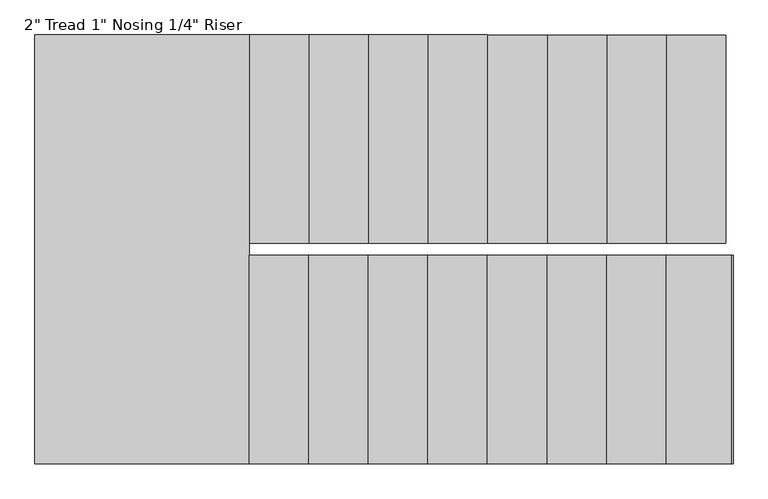
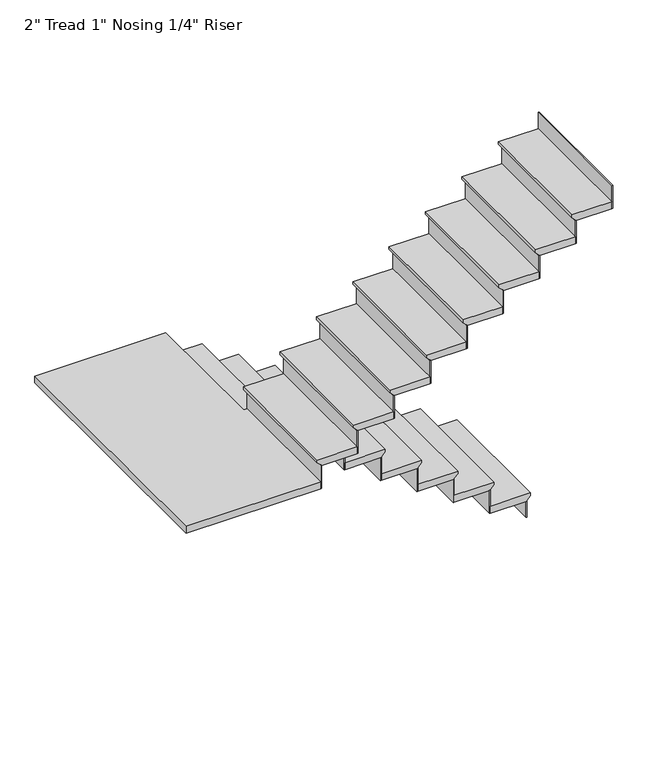
"""IFC4 building model written with IfcOpenShell, lengths in millimetres: stair flight geometry."""

from ifc_helpers import new_model, si_unit, origin, place, context, project, spatial, faceted_brep, source, transform, mapped, element, save


def stair_flight_417d3b76(model_context):
    return source(origin(), model_context, "Body", "Brep", [
        faceted_brep([(-2748.0012202, 5930.6309003, 9294.2833333), (-2748.0012202, 5930.6309003, 9313.3333333), (-2748.0012202, 5041.6309003, 9313.3333333), (-2748.0012202, 5041.6309003, 9294.2833333), (-2773.4012202, 5930.6309003, 9268.8833333), (-2773.4012202, 5041.6309003, 9268.8833333), (-3027.4012202, 5930.6309003, 9313.3333333), (-3027.4012202, 5041.6309003, 9313.3333333), (-2773.4012202, 5041.6309003, 9262.5333333), (-3027.4012202, 5041.6309003, 9262.5333333), (-3027.4012202, 5930.6309003, 9262.5333333), (-2773.4012202, 5930.6309003, 9262.5333333)], [[[0, 1, 2, 3]], [[4, 0, 3, 5]], [[2, 1, 6, 7]], [[8, 9, 10, 11]], [[2, 7, 9, 8, 5, 3]], [[8, 11, 4, 5]], [[6, 1, 0, 4, 11, 10]], [[7, 6, 10, 9]]]),
        faceted_brep([(-2773.4012202, 5930.6309003, 9262.5333333), (-2773.4012202, 5930.6309003, 9144.0), (-2779.7512202, 5930.6309003, 9144.0), (-2779.7512202, 5930.6309003, 9262.5333333), (-2773.4012202, 5041.6309003, 9262.5333333), (-2779.7512202, 5041.6309003, 9262.5333333), (-2779.7512202, 5041.6309003, 9144.0), (-2773.4012202, 5041.6309003, 9144.0)], [[[0, 1, 2, 3]], [[4, 5, 6, 7]], [[1, 0, 4, 7]], [[2, 1, 7, 6]], [[3, 2, 6, 5]], [[0, 3, 5, 4]]]),
        faceted_brep([(-3027.4012202, 5930.6309003, 9431.8666667), (-3027.4012202, 5930.6309003, 9262.5333333), (-3033.7512202, 5930.6309003, 9262.5333333), (-3033.7512202, 5930.6309003, 9431.8666667), (-3027.4012202, 5041.6309003, 9431.8666667), (-3033.7512202, 5041.6309003, 9431.8666667), (-3033.7512202, 5041.6309003, 9262.5333333), (-3027.4012202, 5041.6309003, 9262.5333333)], [[[0, 1, 2, 3]], [[4, 5, 6, 7]], [[1, 0, 4, 7]], [[2, 1, 7, 6]], [[3, 2, 6, 5]], [[0, 3, 5, 4]]]),
        faceted_brep([(-3002.0012202, 5041.6309003, 9482.6666667), (-3002.0012202, 5930.6309003, 9482.6666667), (-3281.4012202, 5930.6309003, 9482.6666667), (-3281.4012202, 5041.6309003, 9482.6666667), (-3027.4012202, 5041.6309003, 9431.8666667), (-3281.4012202, 5041.6309003, 9431.8666667), (-3281.4012202, 5930.6309003, 9431.8666667), (-3027.4012202, 5930.6309003, 9431.8666667), (-3027.4012202, 5041.6309003, 9438.2166667), (-3002.0012202, 5041.6309003, 9463.6166667), (-3027.4012202, 5930.6309003, 9438.2166667), (-3002.0012202, 5930.6309003, 9463.6166667)], [[[0, 1, 2, 3]], [[4, 5, 6, 7]], [[0, 3, 5, 4, 8, 9]], [[4, 7, 10, 8]], [[2, 1, 11, 10, 7, 6]], [[3, 2, 6, 5]], [[11, 1, 0, 9]], [[10, 11, 9, 8]]]),
        faceted_brep([(-3281.4012202, 5930.6309003, 9601.2), (-3281.4012202, 5930.6309003, 9431.8666667), (-3287.7512202, 5930.6309003, 9431.8666667), (-3287.7512202, 5930.6309003, 9601.2), (-3281.4012202, 5041.6309003, 9601.2), (-3287.7512202, 5041.6309003, 9601.2), (-3287.7512202, 5041.6309003, 9431.8666667), (-3281.4012202, 5041.6309003, 9431.8666667)], [[[0, 1, 2, 3]], [[4, 5, 6, 7]], [[1, 0, 4, 7]], [[2, 1, 7, 6]], [[3, 2, 6, 5]], [[0, 3, 5, 4]]]),
        faceted_brep([(-3256.0012202, 5041.6309003, 9652.0), (-3256.0012202, 5930.6309003, 9652.0), (-3535.4012202, 5930.6309003, 9652.0), (-3535.4012202, 5041.6309003, 9652.0), (-3281.4012202, 5041.6309003, 9601.2), (-3535.4012202, 5041.6309003, 9601.2), (-3535.4012202, 5930.6309003, 9601.2), (-3281.4012202, 5930.6309003, 9601.2), (-3281.4012202, 5041.6309003, 9607.55), (-3256.0012202, 5041.6309003, 9632.95), (-3281.4012202, 5930.6309003, 9607.55), (-3256.0012202, 5930.6309003, 9632.95)], [[[0, 1, 2, 3]], [[4, 5, 6, 7]], [[0, 3, 5, 4, 8, 9]], [[4, 7, 10, 8]], [[2, 1, 11, 10, 7, 6]], [[3, 2, 6, 5]], [[11, 1, 0, 9]], [[10, 11, 9, 8]]]),
        faceted_brep([(-3535.4012202, 5930.6309003, 9770.5333333), (-3535.4012202, 5930.6309003, 9601.2), (-3541.7512202, 5930.6309003, 9601.2), (-3541.7512202, 5930.6309003, 9770.5333333), (-3535.4012202, 5041.6309003, 9770.5333333), (-3541.7512202, 5041.6309003, 9770.5333333), (-3541.7512202, 5041.6309003, 9601.2), (-3535.4012202, 5041.6309003, 9601.2)], [[[0, 1, 2, 3]], [[4, 5, 6, 7]], [[1, 0, 4, 7]], [[2, 1, 7, 6]], [[3, 2, 6, 5]], [[0, 3, 5, 4]]]),
        faceted_brep([(-3510.0012202, 5041.6309003, 9821.3333333), (-3510.0012202, 5930.6309003, 9821.3333333), (-3789.4012202, 5930.6309003, 9821.3333333), (-3789.4012202, 5041.6309003, 9821.3333333), (-3535.4012202, 5041.6309003, 9770.5333333), (-3789.4012202, 5041.6309003, 9770.5333333), (-3789.4012202, 5930.6309003, 9770.5333333), (-3535.4012202, 5930.6309003, 9770.5333333), (-3535.4012202, 5041.6309003, 9776.8833333), (-3510.0012202, 5041.6309003, 9802.2833333), (-3535.4012202, 5930.6309003, 9776.8833333), (-3510.0012202, 5930.6309003, 9802.2833333)], [[[0, 1, 2, 3]], [[4, 5, 6, 7]], [[0, 3, 5, 4, 8, 9]], [[4, 7, 10, 8]], [[2, 1, 11, 10, 7, 6]], [[3, 2, 6, 5]], [[11, 1, 0, 9]], [[10, 11, 9, 8]]]),
        faceted_brep([(-3789.4012202, 5930.6309003, 9939.8666667), (-3789.4012202, 5930.6309003, 9770.5333333), (-3795.7512202, 5930.6309003, 9770.5333333), (-3795.7512202, 5930.6309003, 9939.8666667), (-3789.4012202, 5041.6309003, 9939.8666667), (-3795.7512202, 5041.6309003, 9939.8666667), (-3795.7512202, 5041.6309003, 9770.5333333), (-3789.4012202, 5041.6309003, 9770.5333333)], [[[0, 1, 2, 3]], [[4, 5, 6, 7]], [[1, 0, 4, 7]], [[2, 1, 7, 6]], [[3, 2, 6, 5]], [[0, 3, 5, 4]]]),
        faceted_brep([(-3764.0012202, 5041.6309003, 9990.6666667), (-3764.0012202, 5930.6309003, 9990.6666667), (-4043.4012202, 5930.6309003, 9990.6666667), (-4043.4012202, 5041.6309003, 9990.6666667), (-3789.4012202, 5041.6309003, 9939.8666667), (-4043.4012202, 5041.6309003, 9939.8666667), (-4043.4012202, 5930.6309003, 9939.8666667), (-3789.4012202, 5930.6309003, 9939.8666667), (-3789.4012202, 5041.6309003, 9946.2166667), (-3764.0012202, 5041.6309003, 9971.6166667), (-3789.4012202, 5930.6309003, 9946.2166667), (-3764.0012202, 5930.6309003, 9971.6166667)], [[[0, 1, 2, 3]], [[4, 5, 6, 7]], [[0, 3, 5, 4, 8, 9]], [[4, 7, 10, 8]], [[2, 1, 11, 10, 7, 6]], [[3, 2, 6, 5]], [[11, 1, 0, 9]], [[10, 11, 9, 8]]]),
        faceted_brep([(-4043.4012202, 5930.6309003, 10109.2), (-4043.4012202, 5930.6309003, 9939.8666667), (-4049.7512202, 5930.6309003, 9939.8666667), (-4049.7512202, 5930.6309003, 10109.2), (-4043.4012202, 5041.6309003, 10109.2), (-4049.7512202, 5041.6309003, 10109.2), (-4049.7512202, 5041.6309003, 9939.8666667), (-4043.4012202, 5041.6309003, 9939.8666667)], [[[0, 1, 2, 3]], [[4, 5, 6, 7]], [[1, 0, 4, 7]], [[2, 1, 7, 6]], [[3, 2, 6, 5]], [[0, 3, 5, 4]]]),
        faceted_brep([(-4018.0012202, 5041.6309003, 10160.0), (-4018.0012202, 5930.6309003, 10160.0), (-4297.4012202, 5930.6309003, 10160.0), (-4297.4012202, 5041.6309003, 10160.0), (-4043.4012202, 5041.6309003, 10109.2), (-4297.4012202, 5041.6309003, 10109.2), (-4297.4012202, 5930.6309003, 10109.2), (-4043.4012202, 5930.6309003, 10109.2), (-4043.4012202, 5041.6309003, 10115.55), (-4018.0012202, 5041.6309003, 10140.95), (-4043.4012202, 5930.6309003, 10115.55), (-4018.0012202, 5930.6309003, 10140.95)], [[[0, 1, 2, 3]], [[4, 5, 6, 7]], [[0, 3, 5, 4, 8, 9]], [[4, 7, 10, 8]], [[2, 1, 11, 10, 7, 6]], [[3, 2, 6, 5]], [[11, 1, 0, 9]], [[10, 11, 9, 8]]]),
        faceted_brep([(-4297.4012202, 5930.6309003, 10278.5333333), (-4297.4012202, 5930.6309003, 10109.2), (-4303.7512202, 5930.6309003, 10109.2), (-4303.7512202, 5930.6309003, 10278.5333333), (-4297.4012202, 5041.6309003, 10278.5333333), (-4303.7512202, 5041.6309003, 10278.5333333), (-4303.7512202, 5041.6309003, 10109.2), (-4297.4012202, 5041.6309003, 10109.2)], [[[0, 1, 2, 3]], [[4, 5, 6, 7]], [[1, 0, 4, 7]], [[2, 1, 7, 6]], [[3, 2, 6, 5]], [[0, 3, 5, 4]]]),
        faceted_brep([(-4272.0012202, 5041.6309003, 10329.3333333), (-4272.0012202, 5930.6309003, 10329.3333333), (-4551.4012202, 5930.6309003, 10329.3333333), (-4551.4012202, 5041.6309003, 10329.3333333), (-4297.4012202, 5041.6309003, 10278.5333333), (-4551.4012202, 5041.6309003, 10278.5333333), (-4551.4012202, 5930.6309003, 10278.5333333), (-4297.4012202, 5930.6309003, 10278.5333333), (-4297.4012202, 5041.6309003, 10284.8833333), (-4272.0012202, 5041.6309003, 10310.2833333), (-4297.4012202, 5930.6309003, 10284.8833333), (-4272.0012202, 5930.6309003, 10310.2833333)], [[[0, 1, 2, 3]], [[4, 5, 6, 7]], [[0, 3, 5, 4, 8, 9]], [[4, 7, 10, 8]], [[2, 1, 11, 10, 7, 6]], [[3, 2, 6, 5]], [[11, 1, 0, 9]], [[10, 11, 9, 8]]]),
        faceted_brep([(-4551.4012202, 5930.6309003, 10447.8666667), (-4551.4012202, 5930.6309003, 10278.5333333), (-4557.7512202, 5930.6309003, 10278.5333333), (-4557.7512202, 5930.6309003, 10447.8666667), (-4551.4012202, 5041.6309003, 10447.8666667), (-4557.7512202, 5041.6309003, 10447.8666667), (-4557.7512202, 5041.6309003, 10278.5333333), (-4551.4012202, 5041.6309003, 10278.5333333)], [[[0, 1, 2, 3]], [[4, 5, 6, 7]], [[1, 0, 4, 7]], [[2, 1, 7, 6]], [[3, 2, 6, 5]], [[0, 3, 5, 4]]]),
        faceted_brep([(-4526.0012202, 5041.6309003, 10498.6666667), (-4526.0012202, 5930.6309003, 10498.6666667), (-4805.4012202, 5930.6309003, 10498.6666667), (-4805.4012202, 5041.6309003, 10498.6666667), (-4551.4012202, 5041.6309003, 10447.8666667), (-4805.4012202, 5041.6309003, 10447.8666667), (-4805.4012202, 5930.6309003, 10447.8666667), (-4551.4012202, 5930.6309003, 10447.8666667), (-4551.4012202, 5041.6309003, 10454.2166667), (-4526.0012202, 5041.6309003, 10479.6166667), (-4551.4012202, 5930.6309003, 10454.2166667), (-4526.0012202, 5930.6309003, 10479.6166667)], [[[0, 1, 2, 3]], [[4, 5, 6, 7]], [[0, 3, 5, 4, 8, 9]], [[4, 7, 10, 8]], [[2, 1, 11, 10, 7, 6]], [[3, 2, 6, 5]], [[11, 1, 0, 9]], [[10, 11, 9, 8]]]),
        faceted_brep([(-4805.4012202, 5930.6309003, 10617.2), (-4805.4012202, 5930.6309003, 10447.8666667), (-4811.7512202, 5930.6309003, 10447.8666667), (-4811.7512202, 5930.6309003, 10617.2), (-4805.4012202, 5041.6309003, 10617.2), (-4811.7512202, 5041.6309003, 10617.2), (-4811.7512202, 5041.6309003, 10447.8666667), (-4805.4012202, 5041.6309003, 10447.8666667)], [[[0, 1, 2, 3]], [[4, 5, 6, 7]], [[1, 0, 4, 7]], [[2, 1, 7, 6]], [[3, 2, 6, 5]], [[0, 3, 5, 4]]]),
        faceted_brep([(-4754.6012202, 4990.8309003, 10668.0), (-4780.0012202, 4990.8309003, 10668.0), (-4780.0012202, 5930.6309003, 10668.0), (-5694.4012202, 5930.6309003, 10668.0), (-5694.4012202, 4101.8309003, 10668.0), (-4754.6012202, 4101.8309003, 10668.0), (-4780.0012202, 4990.8309003, 10617.2), (-4754.6012202, 4990.8309003, 10617.2), (-4754.6012202, 4101.8309003, 10617.2), (-5694.4012202, 4101.8309003, 10617.2), (-5694.4012202, 5930.6309003, 10617.2), (-4805.4012202, 5930.6309003, 10617.2), (-4805.4012202, 5041.6309003, 10617.2), (-4780.0012202, 5041.6309003, 10617.2), (-4780.0012202, 5041.6309003, 10648.95), (-4780.0012202, 5930.6309003, 10648.95), (-4805.4012202, 5041.6309003, 10623.55), (-4805.4012202, 5930.6309003, 10623.55)], [[[0, 1, 2, 3, 4, 5]], [[6, 7, 8, 9, 10, 11, 12, 13]], [[1, 0, 7, 6]], [[2, 1, 6, 13, 14, 15]], [[13, 12, 16, 14]], [[12, 11, 17, 16]], [[3, 2, 15, 17, 11, 10]], [[4, 3, 10, 9]], [[5, 4, 9, 8]], [[0, 5, 8, 7]], [[17, 15, 14, 16]]]),
        faceted_brep([(-4754.6012202, 4101.8309003, 10786.5333333), (-4754.6012202, 4101.8309003, 10617.2), (-4748.2512202, 4101.8309003, 10617.2), (-4748.2512202, 4101.8309003, 10786.5333333), (-4754.6012202, 4990.8309003, 10786.5333333), (-4748.2512202, 4990.8309003, 10786.5333333), (-4748.2512202, 4990.8309003, 10617.2), (-4754.6012202, 4990.8309003, 10617.2)], [[[0, 1, 2, 3]], [[4, 5, 6, 7]], [[1, 0, 4, 7]], [[2, 1, 7, 6]], [[3, 2, 6, 5]], [[0, 3, 5, 4]]]),
        faceted_brep([(-4780.0012202, 4990.8309003, 10837.3333333), (-4780.0012202, 4101.8309003, 10837.3333333), (-4500.6012202, 4101.8309003, 10837.3333333), (-4500.6012202, 4990.8309003, 10837.3333333), (-4754.6012202, 4990.8309003, 10786.5333333), (-4500.6012202, 4990.8309003, 10786.5333333), (-4500.6012202, 4101.8309003, 10786.5333333), (-4754.6012202, 4101.8309003, 10786.5333333), (-4754.6012202, 4990.8309003, 10792.8833333), (-4780.0012202, 4990.8309003, 10818.2833333), (-4754.6012202, 4101.8309003, 10792.8833333), (-4780.0012202, 4101.8309003, 10818.2833333)], [[[0, 1, 2, 3]], [[4, 5, 6, 7]], [[0, 3, 5, 4, 8, 9]], [[4, 7, 10, 8]], [[2, 1, 11, 10, 7, 6]], [[3, 2, 6, 5]], [[11, 1, 0, 9]], [[10, 11, 9, 8]]]),
        faceted_brep([(-4500.6012202, 4101.8309003, 10955.8666667), (-4500.6012202, 4101.8309003, 10786.5333333), (-4494.2512202, 4101.8309003, 10786.5333333), (-4494.2512202, 4101.8309003, 10955.8666667), (-4500.6012202, 4990.8309003, 10955.8666667), (-4494.2512202, 4990.8309003, 10955.8666667), (-4494.2512202, 4990.8309003, 10786.5333333), (-4500.6012202, 4990.8309003, 10786.5333333)], [[[0, 1, 2, 3]], [[4, 5, 6, 7]], [[1, 0, 4, 7]], [[2, 1, 7, 6]], [[3, 2, 6, 5]], [[0, 3, 5, 4]]]),
        faceted_brep([(-4526.0012202, 4990.8309003, 11006.6666667), (-4526.0012202, 4101.8309003, 11006.6666667), (-4246.6012202, 4101.8309003, 11006.6666667), (-4246.6012202, 4990.8309003, 11006.6666667), (-4500.6012202, 4990.8309003, 10955.8666667), (-4246.6012202, 4990.8309003, 10955.8666667), (-4246.6012202, 4101.8309003, 10955.8666667), (-4500.6012202, 4101.8309003, 10955.8666667), (-4500.6012202, 4990.8309003, 10962.2166667), (-4526.0012202, 4990.8309003, 10987.6166667), (-4500.6012202, 4101.8309003, 10962.2166667), (-4526.0012202, 4101.8309003, 10987.6166667)], [[[0, 1, 2, 3]], [[4, 5, 6, 7]], [[0, 3, 5, 4, 8, 9]], [[4, 7, 10, 8]], [[2, 1, 11, 10, 7, 6]], [[3, 2, 6, 5]], [[11, 1, 0, 9]], [[10, 11, 9, 8]]]),
        faceted_brep([(-4246.6012202, 4101.8309003, 11125.2), (-4246.6012202, 4101.8309003, 10955.8666667), (-4240.2512202, 4101.8309003, 10955.8666667), (-4240.2512202, 4101.8309003, 11125.2), (-4246.6012202, 4990.8309003, 11125.2), (-4240.2512202, 4990.8309003, 11125.2), (-4240.2512202, 4990.8309003, 10955.8666667), (-4246.6012202, 4990.8309003, 10955.8666667)], [[[0, 1, 2, 3]], [[4, 5, 6, 7]], [[1, 0, 4, 7]], [[2, 1, 7, 6]], [[3, 2, 6, 5]], [[0, 3, 5, 4]]]),
        faceted_brep([(-4272.0012202, 4990.8309003, 11176.0), (-4272.0012202, 4101.8309003, 11176.0), (-3992.6012202, 4101.8309003, 11176.0), (-3992.6012202, 4990.8309003, 11176.0), (-4246.6012202, 4990.8309003, 11125.2), (-3992.6012202, 4990.8309003, 11125.2), (-3992.6012202, 4101.8309003, 11125.2), (-4246.6012202, 4101.8309003, 11125.2), (-4246.6012202, 4990.8309003, 11131.55), (-4272.0012202, 4990.8309003, 11156.95), (-4246.6012202, 4101.8309003, 11131.55), (-4272.0012202, 4101.8309003, 11156.95)], [[[0, 1, 2, 3]], [[4, 5, 6, 7]], [[0, 3, 5, 4, 8, 9]], [[4, 7, 10, 8]], [[2, 1, 11, 10, 7, 6]], [[3, 2, 6, 5]], [[11, 1, 0, 9]], [[10, 11, 9, 8]]]),
        faceted_brep([(-3992.6012202, 4101.8309003, 11294.5333333), (-3992.6012202, 4101.8309003, 11125.2), (-3986.2512202, 4101.8309003, 11125.2), (-3986.2512202, 4101.8309003, 11294.5333333), (-3992.6012202, 4990.8309003, 11294.5333333), (-3986.2512202, 4990.8309003, 11294.5333333), (-3986.2512202, 4990.8309003, 11125.2), (-3992.6012202, 4990.8309003, 11125.2)], [[[0, 1, 2, 3]], [[4, 5, 6, 7]], [[1, 0, 4, 7]], [[2, 1, 7, 6]], [[3, 2, 6, 5]], [[0, 3, 5, 4]]]),
        faceted_brep([(-4018.0012202, 4990.8309003, 11345.3333333), (-4018.0012202, 4101.8309003, 11345.3333333), (-3738.6012202, 4101.8309003, 11345.3333333), (-3738.6012202, 4990.8309003, 11345.3333333), (-3992.6012202, 4990.8309003, 11294.5333333), (-3738.6012202, 4990.8309003, 11294.5333333), (-3738.6012202, 4101.8309003, 11294.5333333), (-3992.6012202, 4101.8309003, 11294.5333333), (-3992.6012202, 4990.8309003, 11300.8833333), (-4018.0012202, 4990.8309003, 11326.2833333), (-3992.6012202, 4101.8309003, 11300.8833333), (-4018.0012202, 4101.8309003, 11326.2833333)], [[[0, 1, 2, 3]], [[4, 5, 6, 7]], [[0, 3, 5, 4, 8, 9]], [[4, 7, 10, 8]], [[2, 1, 11, 10, 7, 6]], [[3, 2, 6, 5]], [[11, 1, 0, 9]], [[10, 11, 9, 8]]]),
        faceted_brep([(-3738.6012202, 4101.8309003, 11463.8666667), (-3738.6012202, 4101.8309003, 11294.5333333), (-3732.2512202, 4101.8309003, 11294.5333333), (-3732.2512202, 4101.8309003, 11463.8666667), (-3738.6012202, 4990.8309003, 11463.8666667), (-3732.2512202, 4990.8309003, 11463.8666667), (-3732.2512202, 4990.8309003, 11294.5333333), (-3738.6012202, 4990.8309003, 11294.5333333)], [[[0, 1, 2, 3]], [[4, 5, 6, 7]], [[1, 0, 4, 7]], [[2, 1, 7, 6]], [[3, 2, 6, 5]], [[0, 3, 5, 4]]]),
        faceted_brep([(-3764.0012202, 4990.8309003, 11514.6666667), (-3764.0012202, 4101.8309003, 11514.6666667), (-3484.6012202, 4101.8309003, 11514.6666667), (-3484.6012202, 4990.8309003, 11514.6666667), (-3738.6012202, 4990.8309003, 11463.8666667), (-3484.6012202, 4990.8309003, 11463.8666667), (-3484.6012202, 4101.8309003, 11463.8666667), (-3738.6012202, 4101.8309003, 11463.8666667), (-3738.6012202, 4990.8309003, 11470.2166667), (-3764.0012202, 4990.8309003, 11495.6166667), (-3738.6012202, 4101.8309003, 11470.2166667), (-3764.0012202, 4101.8309003, 11495.6166667)], [[[0, 1, 2, 3]], [[4, 5, 6, 7]], [[0, 3, 5, 4, 8, 9]], [[4, 7, 10, 8]], [[2, 1, 11, 10, 7, 6]], [[3, 2, 6, 5]], [[11, 1, 0, 9]], [[10, 11, 9, 8]]]),
        faceted_brep([(-3484.6012202, 4101.8309003, 11633.2), (-3484.6012202, 4101.8309003, 11463.8666667), (-3478.2512202, 4101.8309003, 11463.8666667), (-3478.2512202, 4101.8309003, 11633.2), (-3484.6012202, 4990.8309003, 11633.2), (-3478.2512202, 4990.8309003, 11633.2), (-3478.2512202, 4990.8309003, 11463.8666667), (-3484.6012202, 4990.8309003, 11463.8666667)], [[[0, 1, 2, 3]], [[4, 5, 6, 7]], [[1, 0, 4, 7]], [[2, 1, 7, 6]], [[3, 2, 6, 5]], [[0, 3, 5, 4]]]),
        faceted_brep([(-3510.0012202, 4990.8309003, 11684.0), (-3510.0012202, 4101.8309003, 11684.0), (-3230.6012202, 4101.8309003, 11684.0), (-3230.6012202, 4990.8309003, 11684.0), (-3484.6012202, 4990.8309003, 11633.2), (-3230.6012202, 4990.8309003, 11633.2), (-3230.6012202, 4101.8309003, 11633.2), (-3484.6012202, 4101.8309003, 11633.2), (-3484.6012202, 4990.8309003, 11639.55), (-3510.0012202, 4990.8309003, 11664.95), (-3484.6012202, 4101.8309003, 11639.55), (-3510.0012202, 4101.8309003, 11664.95)], [[[0, 1, 2, 3]], [[4, 5, 6, 7]], [[0, 3, 5, 4, 8, 9]], [[4, 7, 10, 8]], [[2, 1, 11, 10, 7, 6]], [[3, 2, 6, 5]], [[11, 1, 0, 9]], [[10, 11, 9, 8]]]),
        faceted_brep([(-3230.6012202, 4101.8309003, 11802.5333333), (-3230.6012202, 4101.8309003, 11633.2), (-3224.2512202, 4101.8309003, 11633.2), (-3224.2512202, 4101.8309003, 11802.5333333), (-3230.6012202, 4990.8309003, 11802.5333333), (-3224.2512202, 4990.8309003, 11802.5333333), (-3224.2512202, 4990.8309003, 11633.2), (-3230.6012202, 4990.8309003, 11633.2)], [[[0, 1, 2, 3]], [[4, 5, 6, 7]], [[1, 0, 4, 7]], [[2, 1, 7, 6]], [[3, 2, 6, 5]], [[0, 3, 5, 4]]]),
        faceted_brep([(-3256.0012202, 4990.8309003, 11853.3333333), (-3256.0012202, 4101.8309003, 11853.3333333), (-2976.6012202, 4101.8309003, 11853.3333333), (-2976.6012202, 4990.8309003, 11853.3333333), (-3230.6012202, 4990.8309003, 11802.5333333), (-2976.6012202, 4990.8309003, 11802.5333333), (-2976.6012202, 4101.8309003, 11802.5333333), (-3230.6012202, 4101.8309003, 11802.5333333), (-3230.6012202, 4990.8309003, 11808.8833333), (-3256.0012202, 4990.8309003, 11834.2833333), (-3230.6012202, 4101.8309003, 11808.8833333), (-3256.0012202, 4101.8309003, 11834.2833333)], [[[0, 1, 2, 3]], [[4, 5, 6, 7]], [[0, 3, 5, 4, 8, 9]], [[4, 7, 10, 8]], [[2, 1, 11, 10, 7, 6]], [[3, 2, 6, 5]], [[11, 1, 0, 9]], [[10, 11, 9, 8]]]),
        faceted_brep([(-2976.6012202, 4101.8309003, 11971.8666667), (-2976.6012202, 4101.8309003, 11802.5333333), (-2970.2512202, 4101.8309003, 11802.5333333), (-2970.2512202, 4101.8309003, 11971.8666667), (-2976.6012202, 4990.8309003, 11971.8666667), (-2970.2512202, 4990.8309003, 11971.8666667), (-2970.2512202, 4990.8309003, 11802.5333333), (-2976.6012202, 4990.8309003, 11802.5333333)], [[[0, 1, 2, 3]], [[4, 5, 6, 7]], [[1, 0, 4, 7]], [[2, 1, 7, 6]], [[3, 2, 6, 5]], [[0, 3, 5, 4]]]),
        faceted_brep([(-2722.6012202, 4101.8309003, 12141.2), (-2722.6012202, 4101.8309003, 11971.8666667), (-2716.2512202, 4101.8309003, 11971.8666667), (-2716.2512202, 4101.8309003, 12141.2), (-2722.6012202, 4990.8309003, 12141.2), (-2716.2512202, 4990.8309003, 12141.2), (-2716.2512202, 4990.8309003, 11971.8666667), (-2722.6012202, 4990.8309003, 11971.8666667)], [[[0, 1, 2, 3]], [[4, 5, 6, 7]], [[1, 0, 4, 7]], [[2, 1, 7, 6]], [[3, 2, 6, 5]], [[0, 3, 5, 4]]]),
        faceted_brep([(-3002.0012202, 4990.8309003, 12022.6666667), (-3002.0012202, 4101.8309003, 12022.6666667), (-2722.6012202, 4101.8309003, 12022.6666667), (-2722.6012202, 4990.8309003, 12022.6666667), (-2976.6012202, 4990.8309003, 11971.8666667), (-2722.6012202, 4990.8309003, 11971.8666667), (-2722.6012202, 4101.8309003, 11971.8666667), (-2976.6012202, 4101.8309003, 11971.8666667), (-2976.6012202, 4990.8309003, 11978.2166667), (-3002.0012202, 4990.8309003, 12003.6166667), (-2976.6012202, 4101.8309003, 11978.2166667), (-3002.0012202, 4101.8309003, 12003.6166667)], [[[0, 1, 2, 3]], [[4, 5, 6, 7]], [[0, 3, 5, 4, 8, 9]], [[4, 7, 10, 8]], [[2, 1, 11, 10, 7, 6]], [[3, 2, 6, 5]], [[11, 1, 0, 9]], [[10, 11, 9, 8]]]),
    ])


if __name__ == "__main__":
    model = new_model("IFC4")
    model_context = context("Model", 3, world=origin())
    ifc_project = project(units=[si_unit("LENGTHUNIT", "METRE", prefix="MILLI")], contexts=[model_context])
    site = spatial("IfcSite", under=ifc_project)
    building = spatial("IfcBuilding", under=site)
    placement = place(None, origin())
    stair_flight_shape = stair_flight_417d3b76(model_context)
    element("IfcStairFlight", 1, ObjectType="2\" Tread 1\" Nosing 1/4\" Riser", at=placement, inside=building, context=model_context, shape_type="MappedRepresentation", body=[
        mapped(stair_flight_shape, transform((0.0, 0.0, 0.0), x_axis=(1.0, 0.0, 0.0), y_axis=(0.0, 1.0, 0.0), z_axis=(0.0, 0.0, 1.0))),
    ])
    save(model, "model.ifc")
